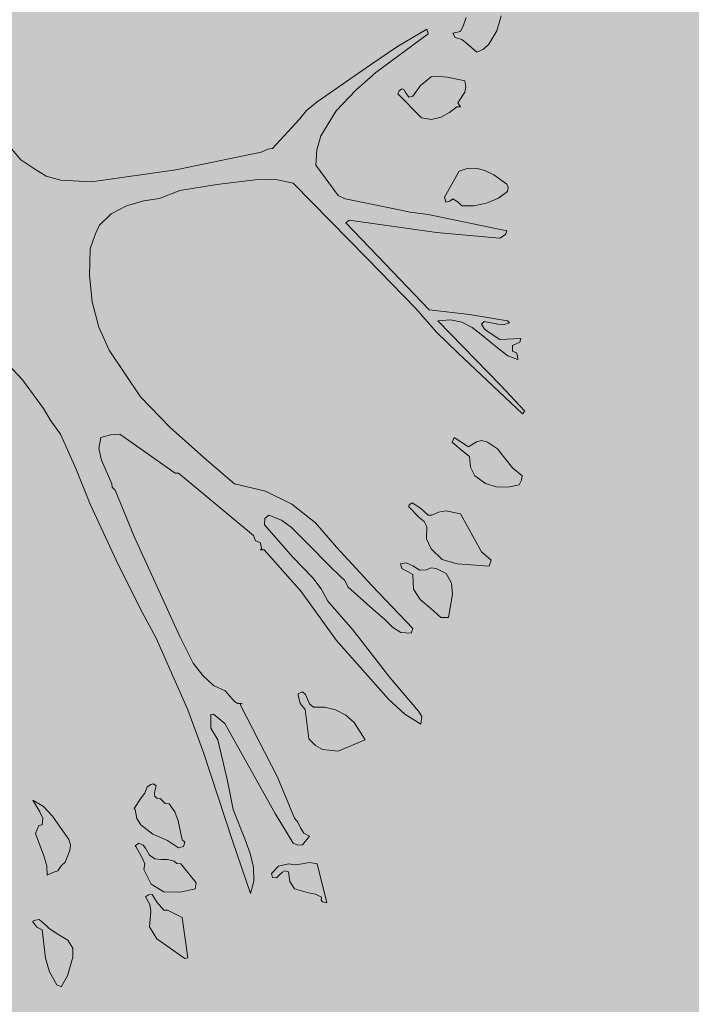
# Model space of a CAD drawing. Units: inches. Extents: x 84 to 1044, y -280 to 906.
# Tile 84 of 105: x 844.48 to 855.93, y 408.65 to 425.45. Entities that reach past the tile are written whole.
import ezdxf

# ---------------------------------------------------------------- set-up
doc = ezdxf.new("R2010")
doc.units = ezdxf.units.IN
doc.layers.add('A-ANNO-DIMS', color=2, linetype='Continuous', lineweight=18)
doc.layers.add('L-PLNT', color=114, linetype='Continuous', lineweight=15)
doc.layers.add('L-PLNT-PATT', color=9, linetype='Continuous', lineweight=9, true_color=0xafd9aa)
doc.styles.get("Standard").update_dxf_attribs({"font": 'arial.ttf'})
doc.dimstyles.get("Standard").update_dxf_attribs({"dimtxt": 0.18, "dimasz": 0.18, "dimexe": 0.18, "dimexo": 0.0625, "dimgap": 0.09, "dimtad": 0, "dimtih": 1, "dimtoh": 1, "dimdec": 4, "dimzin": 0, "dimdsep": 46, "dimtxsty": 'Standard', "dimcen": 0.09, "dimadec": 0, "dimazin": 0, "dimtfac": 1, "dimtdec": 4, "dimtofl": 0, "dimtmove": 0, "dimatfit": 3, "dimfxl": 1, "dimtolj": 1, "dimtzin": 0, "dimarcsym": 0})

# ---------------------------------------------------------------- blocks, each defined once
blk = doc.blocks.new('A$C37E508DF')
for p, q in [((1.3455, 1.0934), (1.3485, 1.102)), ((1.3875, 1.1037), (1.3828, 1.087)), ((1.3057, 1.0835), (1.2469, 1.0402)), ((1.2713, 1.0694), (1.3044, 1.0887)), ((1.3044, 1.0887), (1.3057, 1.0835)), ((1.3335, 1.0844), (1.3421, 1.0861)), ((1.3361, 1.0793), (1.3335, 1.0844)), ((1.3421, 1.0861), (1.3455, 1.0934)), ((1.3828, 1.087), (1.3738, 1.072)), ((1.3434, 1.0771), (1.3361, 1.0793)), ((1.349, 1.0728), (1.3434, 1.0771)), ((1.3605, 1.063), (1.349, 1.0728)), ((1.2409, 1.0488), (1.2713, 1.0694)), ((1.3678, 1.0664), (1.3605, 1.063)), ((1.3738, 1.072), (1.3678, 1.0664)), ((1.1813, 1.0072), (1.2409, 1.0488)), ((1.2469, 1.0402), (1.2246, 1.0201)), ((1.2971, 1.0257), (1.3091, 1.0351)), ((1.3091, 1.0351), (1.3185, 1.0355)), ((1.3185, 1.0355), (1.3275, 1.0347)), ((1.3275, 1.0347), (1.3468, 1.0308)), ((1.3468, 1.0308), (1.3481, 1.0239)), ((1.2246, 1.0201), (1.2023, 0.9969)), ((1.2718, 1.0162), (1.2731, 1.0197)), ((1.2731, 1.0197), (1.2761, 1.0218)), ((1.2761, 1.0218), (1.2786, 1.0209)), ((1.2786, 1.0209), (1.2799, 1.0184)), ((1.2799, 1.0184), (1.2842, 1.0124)), ((1.2885, 1.0136), (1.2971, 1.0257)), ((1.3468, 1.018), (1.3391, 1.0059)), ((1.3481, 1.0239), (1.3468, 1.018)), ((1.1693, 0.9974), (1.1813, 1.0072)), ((1.2984, 0.9892), (1.2718, 1.0162)), ((1.2842, 1.0124), (1.2885, 1.0136)), ((1.3391, 1.0059), (1.3421, 1.0016)), ((1.1612, 0.9879), (1.1693, 0.9974)), ((1.2023, 0.9969), (1.1852, 0.9691)), ((1.3297, 0.9952), (1.3202, 0.9901)), ((1.3378, 1.0016), (1.3297, 0.9952)), ((1.3421, 1.0016), (1.3378, 1.0016)), ((1.1311, 0.9549), (1.1612, 0.9879)), ((1.3095, 0.9875), (1.2984, 0.9892)), ((1.3202, 0.9901), (1.3095, 0.9875)), ((1.1852, 0.9691), (1.1809, 0.9532)), ((0.8383, 0.954), (0.8486, 0.942)), ((1.0227, 0.9309), (1.1183, 0.9506)), ((1.1183, 0.9506), (1.1256, 0.954)), ((1.1256, 0.954), (1.1311, 0.9549)), ((1.1809, 0.9532), (1.1796, 0.936)), ((0.8486, 0.942), (0.8619, 0.933)), ((0.8619, 0.933), (0.8769, 0.9236)), ((0.9279, 0.9172), (1.0227, 0.9309)), ((1.1796, 0.936), (1.2049, 0.9022)), ((1.3241, 0.9), (1.3404, 0.9292)), ((1.3404, 0.9292), (1.3494, 0.9322)), ((1.3494, 0.9322), (1.3592, 0.9326)), ((1.3592, 0.9326), (1.3695, 0.93)), ((1.3695, 0.93), (1.3794, 0.9253)), ((0.8769, 0.9236), (0.8936, 0.9193)), ((0.8936, 0.9193), (0.9279, 0.9172)), ((1.1114, 0.9198), (1.0685, 0.9142)), ((1.1333, 0.9202), (1.1114, 0.9198)), ((1.1543, 0.9159), (1.1333, 0.9202)), ((1.3794, 0.9253), (1.394, 0.9146)), ((1.0269, 0.9077), (1.0042, 0.8987)), ((1.0685, 0.9142), (1.0269, 0.9077)), ((1.2371, 0.8314), (1.1543, 0.9159)), ((1.3948, 0.9065), (1.3846, 0.8992)), ((1.394, 0.9146), (1.3957, 0.9112)), ((1.3957, 0.9112), (1.3948, 0.9065)), ((0.9866, 0.8962), (0.9673, 0.8906)), ((1.0042, 0.8987), (0.9866, 0.8962)), ((1.2049, 0.9022), (1.2126, 0.8983)), ((1.2126, 0.8983), (1.2662, 0.8876)), ((1.3254, 0.8944), (1.3241, 0.9)), ((1.3301, 0.8957), (1.3254, 0.8944)), ((1.3335, 0.8983), (1.3301, 0.8957)), ((1.3395, 0.8944), (1.3335, 0.8983)), ((1.3846, 0.8992), (1.3713, 0.8936)), ((0.9673, 0.8906), (0.9498, 0.8816)), ((1.2662, 0.8876), (1.2855, 0.8833)), ((1.3434, 0.8906), (1.3395, 0.8944)), ((1.3571, 0.8906), (1.3434, 0.8906)), ((1.3713, 0.8936), (1.3571, 0.8906)), ((0.9498, 0.8816), (0.9369, 0.8687)), ((1.2169, 0.8743), (1.2135, 0.8713)), ((1.3151, 0.8606), (1.2169, 0.8743)), ((1.2855, 0.8833), (1.3057, 0.8807)), ((1.3057, 0.8807), (1.394, 0.8623)), ((0.9369, 0.8687), (0.933, 0.861)), ((1.2135, 0.8713), (1.2491, 0.834)), ((1.394, 0.8623), (1.3927, 0.8584)), ((0.9296, 0.852), (0.9262, 0.8421)), ((0.933, 0.861), (0.9296, 0.852)), ((1.3863, 0.8541), (1.3151, 0.8606)), ((1.3927, 0.8584), (1.3863, 0.8541)), ((0.9262, 0.8421), (0.9257, 0.8121)), ((1.2919, 0.7752), (1.2371, 0.8314)), ((1.2491, 0.834), (1.3069, 0.7735)), ((0.9257, 0.8121), (0.9287, 0.7825)), ((0.9287, 0.7825), (0.936, 0.7542)), ((1.3151, 0.7487), (1.2919, 0.7752)), ((1.3069, 0.7735), (1.352, 0.7684)), ((1.352, 0.7684), (1.3948, 0.7615)), ((0.936, 0.7542), (0.9476, 0.7285)), ((1.3309, 0.7624), (1.3164, 0.7615)), ((1.3164, 0.7615), (1.3871, 0.6891)), ((1.3434, 0.7598), (1.3309, 0.7624)), ((1.355, 0.7538), (1.3434, 0.7598)), ((1.3653, 0.7461), (1.355, 0.7538)), ((1.3687, 0.7607), (1.3657, 0.7577)), ((1.3657, 0.7577), (1.3691, 0.7521)), ((1.3841, 0.7577), (1.3687, 0.7607)), ((1.3691, 0.7521), (1.3743, 0.7482)), ((1.3914, 0.7572), (1.3841, 0.7577)), ((1.397, 0.759), (1.3914, 0.7572)), ((1.3948, 0.7615), (1.397, 0.759)), ((1.3391, 0.7255), (1.3151, 0.7487)), ((1.3854, 0.7294), (1.3653, 0.7461)), ((1.3743, 0.7482), (1.3863, 0.7405)), ((1.3863, 0.7405), (1.4099, 0.7414)), ((1.4099, 0.7414), (1.4086, 0.7375)), ((1.4086, 0.7375), (1.4004, 0.7337)), ((1.4004, 0.7337), (1.4004, 0.7272)), ((0.9476, 0.7285), (0.9828, 0.6762)), ((1.4116, 0.6569), (1.3391, 0.7255)), ((1.3953, 0.7221), (1.3854, 0.7294)), ((1.4064, 0.7178), (1.3953, 0.7221)), ((1.4004, 0.7272), (1.4047, 0.7255)), ((1.4047, 0.7255), (1.406, 0.7221)), ((1.406, 0.7221), (1.4064, 0.7178)), ((0.8503, 0.6951), (0.8344, 0.7122)), ((0.8739, 0.6629), (0.8503, 0.6951)), ((1.3871, 0.6891), (1.4141, 0.6599)), ((0.9828, 0.6762), (1.0162, 0.6415)), ((0.8824, 0.6492), (0.8739, 0.6629)), ((1.4141, 0.6599), (1.4116, 0.6569)), ((0.8932, 0.6342), (0.8824, 0.6492)), ((1.0162, 0.6415), (1.0574, 0.605)), ((0.9103, 0.5956), (0.8932, 0.6342)), ((0.9382, 0.6303), (0.936, 0.6179)), ((0.9493, 0.6333), (0.9382, 0.6303)), ((0.9596, 0.6342), (0.9493, 0.6333)), ((1.0218, 0.5904), (0.9596, 0.6342)), ((1.3327, 0.6252), (1.3348, 0.6303)), ((1.3348, 0.6303), (1.3511, 0.62)), ((1.343, 0.6162), (1.3327, 0.6252)), ((1.3511, 0.62), (1.3601, 0.6256)), ((1.3601, 0.6256), (1.3661, 0.6269)), ((1.3661, 0.6269), (1.3725, 0.6252)), ((1.3725, 0.6252), (1.3837, 0.6175)), ((0.936, 0.6179), (0.939, 0.605)), ((1.352, 0.6089), (1.343, 0.6162)), ((1.3533, 0.5969), (1.352, 0.6089)), ((1.3837, 0.6175), (1.3918, 0.6072)), ((0.939, 0.605), (0.9506, 0.5784)), ((1.0574, 0.605), (1.0883, 0.5784)), ((1.358, 0.5874), (1.3533, 0.5969)), ((1.3918, 0.6072), (1.4004, 0.5964)), ((0.9262, 0.5557), (0.9103, 0.5956)), ((1.0256, 0.5904), (1.0218, 0.5904)), ((1.1097, 0.5205), (1.0256, 0.5904)), ((1.37, 0.5789), (1.358, 0.5874)), ((1.4004, 0.5964), (1.4111, 0.5874)), ((1.4111, 0.5874), (1.4103, 0.5823)), ((0.9506, 0.5784), (0.951, 0.5746)), ((1.0883, 0.5784), (1.123, 0.5703)), ((1.3824, 0.575), (1.37, 0.5789)), ((1.3953, 0.5746), (1.3824, 0.575)), ((1.4077, 0.5771), (1.3953, 0.5746)), ((1.4103, 0.5823), (1.4077, 0.5771)), ((0.951, 0.5746), (0.9545, 0.5711)), ((0.9545, 0.5711), (0.9759, 0.5193)), ((1.123, 0.5703), (1.1526, 0.5557)), ((0.9583, 0.4871), (0.9262, 0.5557)), ((1.1526, 0.5557), (1.1792, 0.5347)), ((1.2842, 0.554), (1.2855, 0.5557)), ((1.2842, 0.5527), (1.2842, 0.554)), ((1.2958, 0.5407), (1.2842, 0.5527)), ((1.2855, 0.5557), (1.2876, 0.557)), ((1.2876, 0.557), (1.2971, 0.551)), ((1.1268, 0.5433), (1.1226, 0.5394)), ((1.141, 0.5377), (1.1268, 0.5433)), ((1.2971, 0.551), (1.3057, 0.5433)), ((1.3057, 0.5433), (1.3099, 0.5433)), ((1.3099, 0.5433), (1.3172, 0.5467)), ((1.3172, 0.5467), (1.3254, 0.548)), ((1.3254, 0.548), (1.3421, 0.5446)), ((1.3421, 0.5446), (1.3657, 0.5021)), ((1.1226, 0.5394), (1.1221, 0.5325)), ((1.1221, 0.5325), (1.1539, 0.4961)), ((1.1521, 0.5296), (1.141, 0.5377)), ((1.1792, 0.5347), (1.2027, 0.5072)), ((1.3014, 0.536), (1.2958, 0.5407)), ((1.3044, 0.53), (1.3014, 0.536)), ((1.1118, 0.5145), (1.1097, 0.5205)), ((1.1706, 0.5111), (1.1521, 0.5296)), ((1.3039, 0.5167), (1.3044, 0.53)), ((0.9759, 0.5193), (1.0269, 0.4069)), ((1.117, 0.5124), (1.1118, 0.5145)), ((1.1191, 0.5055), (1.117, 0.5124)), ((1.1955, 0.4858), (1.1706, 0.5111)), ((1.3091, 0.5055), (1.3039, 0.5167)), ((1.117, 0.5042), (1.1191, 0.5055)), ((1.1217, 0.5042), (1.117, 0.5042)), ((1.1633, 0.4575), (1.1217, 0.5042)), ((1.2027, 0.5072), (1.2426, 0.4644)), ((1.3215, 0.4935), (1.3091, 0.5055)), ((1.3657, 0.5021), (1.3764, 0.4927)), ((0.9853, 0.4335), (0.9583, 0.4871)), ((1.1539, 0.4961), (1.1762, 0.4729)), ((1.2748, 0.4884), (1.2812, 0.4897)), ((1.2761, 0.4832), (1.2748, 0.4884)), ((1.2812, 0.4897), (1.2885, 0.4862)), ((1.3382, 0.4884), (1.3215, 0.4935)), ((1.3743, 0.4858), (1.3382, 0.4884)), ((1.3764, 0.4927), (1.3743, 0.4858)), ((1.207, 0.4747), (1.1955, 0.4858)), ((1.2825, 0.4798), (1.2761, 0.4832)), ((1.2885, 0.4764), (1.2825, 0.4798)), ((1.2885, 0.4862), (1.2962, 0.4815)), ((1.2894, 0.4601), (1.2885, 0.4764)), ((1.2962, 0.4815), (1.3039, 0.482)), ((1.3039, 0.482), (1.3087, 0.4841)), ((1.3087, 0.4841), (1.3147, 0.4832)), ((1.3147, 0.4832), (1.3258, 0.4777)), ((1.3258, 0.4777), (1.3318, 0.4669)), ((1.1762, 0.4729), (1.1856, 0.4605)), ((1.2122, 0.47), (1.207, 0.4747)), ((1.2156, 0.4627), (1.2122, 0.47)), ((1.2426, 0.4644), (1.2885, 0.4159)), ((1.3318, 0.4669), (1.3331, 0.4545)), ((1.2027, 0.4026), (1.1633, 0.4575)), ((1.1856, 0.4605), (1.1933, 0.4468)), ((1.2469, 0.4348), (1.2156, 0.4627)), ((1.2967, 0.4485), (1.2894, 0.4601)), ((1.3331, 0.4545), (1.3284, 0.4284)), ((1.1933, 0.4468), (1.2212, 0.4146)), ((1.3082, 0.4386), (1.2967, 0.4485)), ((1.0003, 0.4052), (0.9853, 0.4335)), ((1.2568, 0.4266), (1.2469, 0.4348)), ((1.3198, 0.4284), (1.3082, 0.4386)), ((1.2658, 0.4176), (1.2568, 0.4266)), ((1.3284, 0.4284), (1.3198, 0.4284)), ((1.2212, 0.4146), (1.2628, 0.361)), ((1.2752, 0.4116), (1.2658, 0.4176)), ((1.2868, 0.4108), (1.2752, 0.4116)), ((1.2885, 0.4159), (1.2868, 0.4108)), ((1.0145, 0.373), (1.0003, 0.4052)), ((1.0269, 0.4069), (1.0419, 0.3769)), ((1.2289, 0.373), (1.2027, 0.4026)), ((1.0419, 0.3769), (1.0527, 0.3632)), ((1.0359, 0.3246), (1.0145, 0.373)), ((1.2615, 0.3362), (1.2289, 0.373)), ((1.0527, 0.3632), (1.0647, 0.352)), ((1.2628, 0.361), (1.2949, 0.3233)), ((1.0647, 0.352), (1.078, 0.346)), ((1.078, 0.346), (1.0883, 0.334)), ((1.1599, 0.3426), (1.1646, 0.3447)), ((1.1646, 0.3447), (1.168, 0.3417)), ((1.0883, 0.334), (1.0921, 0.3319)), ((1.0921, 0.3319), (1.0968, 0.3319)), ((1.0968, 0.3319), (1.0947, 0.3306)), ((1.1599, 0.3413), (1.1599, 0.3426)), ((1.162, 0.3319), (1.1599, 0.3413)), ((1.1676, 0.325), (1.162, 0.3319)), ((1.168, 0.3417), (1.1702, 0.3366)), ((1.1702, 0.3366), (1.1727, 0.3314)), ((1.2795, 0.3199), (1.2615, 0.3362)), ((1.0535, 0.2766), (1.0359, 0.3246)), ((1.0947, 0.3306), (1.1367, 0.2491)), ((1.1719, 0.292), (1.1676, 0.325)), ((1.1727, 0.3314), (1.177, 0.3276)), ((1.177, 0.3276), (1.1895, 0.3276)), ((1.1895, 0.3276), (1.2019, 0.3246)), ((1.2019, 0.3246), (1.2135, 0.3186)), ((1.2949, 0.3233), (1.2988, 0.3173)), ((1.0647, 0.3199), (1.0617, 0.3194)), ((1.0617, 0.3194), (1.0617, 0.304)), ((1.0711, 0.3147), (1.0647, 0.3199)), ((1.0775, 0.3092), (1.0711, 0.3147)), ((1.2135, 0.3186), (1.2225, 0.3104)), ((1.2225, 0.3104), (1.2349, 0.2911)), ((1.2975, 0.3087), (1.2795, 0.3199)), ((1.2988, 0.3173), (1.2975, 0.3087)), ((1.0617, 0.304), (1.0698, 0.2911)), ((1.1341, 0.2084), (1.0775, 0.3092)), ((1.0698, 0.2911), (1.0805, 0.2448)), ((1.1792, 0.2847), (1.1719, 0.292)), ((1.2349, 0.2911), (1.2049, 0.2783)), ((1.0861, 0.1775), (1.0535, 0.2766)), ((1.1873, 0.28), (1.1792, 0.2847)), ((1.2049, 0.2783), (1.1873, 0.28)), ((1.0805, 0.2448), (1.087, 0.2127)), ((1.1367, 0.2491), (1.1556, 0.2032)), ((0.9879, 0.2311), (0.9905, 0.2384)), ((0.9905, 0.2384), (0.9943, 0.241)), ((0.9943, 0.241), (0.9973, 0.2414)), ((0.9973, 0.2414), (1.0003, 0.2393)), ((1.0003, 0.2393), (0.9986, 0.232)), ((0.8619, 0.2234), (0.8739, 0.2161)), ((0.87, 0.2101), (0.8619, 0.2234)), ((0.9759, 0.214), (0.9836, 0.226)), ((0.9836, 0.226), (0.9879, 0.2311)), ((0.9986, 0.232), (0.9986, 0.2281)), ((0.9986, 0.2281), (1.0012, 0.2255)), ((1.0012, 0.2255), (1.0051, 0.2251)), ((1.0051, 0.2251), (1.0076, 0.2225)), ((1.0076, 0.2225), (1.0106, 0.2195)), ((0.8734, 0.2032), (0.87, 0.2101)), ((0.8739, 0.2161), (0.8841, 0.2054)), ((0.9768, 0.2127), (0.9759, 0.214)), ((0.9789, 0.2028), (0.9768, 0.2127)), ((1.0106, 0.2195), (1.0149, 0.2191)), ((1.0149, 0.2191), (1.0214, 0.2101)), ((1.0214, 0.2101), (1.0252, 0.2002)), ((1.087, 0.2127), (1.0998, 0.1797)), ((0.8726, 0.1955), (0.8734, 0.2032)), ((0.8841, 0.2054), (0.9026, 0.1792)), ((0.9832, 0.1955), (0.9789, 0.2028)), ((1.0252, 0.2002), (1.0295, 0.1788)), ((1.1543, 0.1749), (1.1341, 0.2084)), ((1.1556, 0.2032), (1.1594, 0.1985)), ((0.8649, 0.1857), (0.8687, 0.1947)), ((0.8687, 0.1947), (0.8726, 0.1955)), ((0.9969, 0.1852), (0.9832, 0.1955)), ((1.1594, 0.1985), (1.1624, 0.1921)), ((1.1624, 0.1921), (1.1663, 0.1861)), ((0.8743, 0.1608), (0.8649, 0.1857)), ((0.9026, 0.1792), (0.9043, 0.1732)), ((1.0132, 0.1779), (0.9969, 0.1852)), ((1.0256, 0.1698), (1.0132, 0.1779)), ((1.0295, 0.1788), (1.0325, 0.1762)), ((1.1063, 0.1183), (1.0861, 0.1775)), ((1.0998, 0.1797), (1.1058, 0.1634)), ((1.1727, 0.1827), (1.1646, 0.1732)), ((1.1663, 0.1861), (1.1727, 0.1827)), ((0.9035, 0.1668), (0.8983, 0.1535)), ((0.9043, 0.1732), (0.9035, 0.1668)), ((0.9768, 0.1719), (0.9811, 0.1749)), ((0.9776, 0.1711), (0.9768, 0.1719)), ((0.9853, 0.1578), (0.9776, 0.1711)), ((0.9811, 0.1749), (0.9858, 0.1728)), ((0.9858, 0.1728), (0.9884, 0.1694)), ((0.9884, 0.1694), (0.9931, 0.1616)), ((1.0312, 0.1711), (1.0256, 0.1698)), ((1.0325, 0.1762), (1.0312, 0.1711)), ((1.1594, 0.1728), (1.1543, 0.1749)), ((1.1646, 0.1732), (1.1594, 0.1728)), ((0.8777, 0.1496), (0.8743, 0.1608)), ((0.9879, 0.1518), (0.9853, 0.1578)), ((0.9931, 0.1616), (0.9991, 0.1574)), ((0.9991, 0.1574), (1.0059, 0.1565)), ((1.0059, 0.1565), (1.0132, 0.1565)), ((1.0132, 0.1565), (1.0205, 0.1548)), ((1.0205, 0.1548), (1.0235, 0.1522)), ((1.1058, 0.1634), (1.1097, 0.1475)), ((0.8781, 0.1389), (0.8777, 0.1496)), ((0.8902, 0.1441), (0.8846, 0.1419)), ((0.894, 0.1496), (0.8902, 0.1441)), ((0.8983, 0.1535), (0.894, 0.1496)), ((0.9866, 0.1453), (0.9879, 0.1518)), ((0.9948, 0.1291), (0.9866, 0.1453)), ((1.0235, 0.1522), (1.0282, 0.1518)), ((1.0282, 0.1518), (1.0454, 0.1303)), ((1.1097, 0.1475), (1.1101, 0.1325)), ((1.1298, 0.1411), (1.1376, 0.1492)), ((1.1376, 0.1492), (1.1491, 0.1518)), ((1.1449, 0.1441), (1.1423, 0.1423)), ((1.1491, 0.1428), (1.1449, 0.1441)), ((1.1491, 0.1518), (1.1564, 0.1505)), ((1.1564, 0.1505), (1.1642, 0.1518)), ((1.1642, 0.1518), (1.1727, 0.1531)), ((1.1727, 0.1531), (1.1813, 0.1518)), ((1.1813, 0.1518), (1.192, 0.108)), ((0.8846, 0.1419), (0.8781, 0.1389)), ((1.1311, 0.1364), (1.1298, 0.1411)), ((1.1354, 0.1359), (1.1311, 0.1364)), ((1.1384, 0.1389), (1.1354, 0.1359)), ((1.1423, 0.1423), (1.1384, 0.1389)), ((1.1504, 0.132), (1.1491, 0.1428)), ((1.0089, 0.1205), (0.9948, 0.1291)), ((1.0441, 0.1239), (1.0274, 0.12)), ((1.0454, 0.1303), (1.0441, 0.1239)), ((1.1101, 0.1325), (1.1063, 0.1183)), ((1.1556, 0.1239), (1.1504, 0.132)), ((1.1714, 0.1192), (1.1556, 0.1239)), ((0.9884, 0.1149), (0.9918, 0.117)), ((0.9935, 0.1063), (0.9884, 0.1149)), ((0.9918, 0.117), (0.9961, 0.1175)), ((0.9961, 0.1175), (1.0016, 0.1085)), ((1.0274, 0.12), (1.0089, 0.1205)), ((1.1792, 0.1179), (1.1714, 0.1192)), ((1.186, 0.1145), (1.1792, 0.1179)), ((1.1856, 0.111), (1.186, 0.1145)), ((1.1873, 0.1093), (1.1856, 0.111)), ((0.9943, 0.0982), (0.9935, 0.1063)), ((1.0016, 0.1085), (1.0089, 0.0999)), ((1.0089, 0.0999), (1.0132, 0.0999)), ((1.0132, 0.0999), (1.0295, 0.0917)), ((1.192, 0.108), (1.1873, 0.1093)), ((0.8619, 0.0875), (0.8649, 0.0887)), ((0.8649, 0.0887), (0.8691, 0.0892)), ((0.8691, 0.0892), (0.8769, 0.0827)), ((0.9931, 0.081), (0.9943, 0.0982)), ((1.0295, 0.0917), (1.0359, 0.0463)), ((0.8619, 0.0866), (0.8619, 0.0875)), ((0.8666, 0.0806), (0.8619, 0.0866)), ((0.8726, 0.0776), (0.8666, 0.0806)), ((0.8764, 0.0459), (0.8726, 0.0776)), ((0.8769, 0.0827), (0.8799, 0.0797)), ((0.8799, 0.0797), (0.8893, 0.0733)), ((1.0012, 0.0677), (0.9931, 0.081)), ((0.8893, 0.0733), (0.9013, 0.066)), ((1.0325, 0.0454), (1.0012, 0.0677)), ((0.9013, 0.066), (0.9069, 0.057)), ((0.9069, 0.057), (0.9069, 0.0471)), ((0.8807, 0.0304), (0.8764, 0.0459)), ((0.9069, 0.0471), (0.9009, 0.0261)), ((1.0359, 0.0463), (1.0325, 0.0454)), ((0.8889, 0.0159), (0.8807, 0.0304)), ((0.9009, 0.0261), (0.894, 0.0137)), ((0.894, 0.0137), (0.8889, 0.0159))]:
    blk.add_line(p, q)
blk = doc.blocks.new('*D62')
at = {"layer": 'A-ANNO-DIMS', "color": 0, "lineweight": -2, "transparency": 16777216}
for p, q in [((203.179, 709.183), (203.179, 905.9)), ((896.074, 400.183), (896.074, 905.9)), ((203.359, 905.72), (549.232, 905.72)), ((895.894, 905.72), (550.021, 905.72))]:
    blk.add_line(p, q, dxfattribs=at)
at = {"layer": 'A-ANNO-DIMS', "color": 0, "transparency": 16777216}
for points in [[(203.359, 905.75), (203.359, 905.69), (203.179, 905.72)], [(895.894, 905.75), (895.894, 905.69), (896.074, 905.72)]]:
    blk.add_solid(points, dxfattribs=at)
at = {"layer": 'Defpoints', "color": 0, "transparency": 16777216}
for p in [(896.074, 905.72), (203.179, 709.12), (896.074, 400.12)]:
    blk.add_point(p, dxfattribs=at)
at = {"layer": 'A-ANNO-DIMS', "color": 0, "transparency": 16777216, "insert": (549.627, 905.72), "char_height": 0.18, "attachment_point": 5}
blk.add_mtext('\\A1;692.9', dxfattribs=at)
blk = doc.blocks.new('*D63')
at = {"layer": 'A-ANNO-DIMS', "color": 0, "lineweight": -2, "transparency": 16777216}
for p, q in [((833.136, 709.12), (1043.768, 709.12)), ((1043.588, 708.94), (1043.588, 400.302)), ((1043.588, 91.3), (1043.588, 399.938)), ((896.136, 91.12), (1043.768, 91.12))]:
    blk.add_line(p, q, dxfattribs=at)
at = {"layer": 'A-ANNO-DIMS', "color": 0, "transparency": 16777216}
for points in [[(1043.558, 708.94), (1043.618, 708.94), (1043.588, 709.12)], [(1043.558, 91.3), (1043.618, 91.3), (1043.588, 91.12)]]:
    blk.add_solid(points, dxfattribs=at)
at = {"layer": 'Defpoints', "color": 0, "transparency": 16777216}
for p in [(833.074, 709.12), (1043.588, 709.12), (896.074, 91.12)]:
    blk.add_point(p, dxfattribs=at)
at = {"layer": 'A-ANNO-DIMS', "color": 0, "transparency": 16777216, "insert": (1043.588, 400.12), "char_height": 0.18, "attachment_point": 5}
blk.add_mtext('\\A1;618', dxfattribs=at)

msp = doc.modelspace()

# ---------------------------------------------------------------- hatches: boundary and pattern name
at = {"layer": 'L-PLNT-PATT', "transparency": 33554597}
h = msp.add_hatch(color=256, dxfattribs=at)
h.dxf.hatch_style = 1
h.paths.add_polyline_path([(896.074, 511.12), (704.074, 511.12), (704.074, 491.62), (704.074, 419.62), (704.074, 400.12), (833.074, 400.12), (896.074, 400.12)])

# ---------------------------------------------------------------- block references
at = {"layer": 'L-PLNT', "xscale": 15.19586232982809, "yscale": 15.19586232982809, "zscale": 15.19586232982809}
msp.add_blockref('A$C37E508DF', (831.605, 408.742), dxfattribs=at)

# ---------------------------------------------------------------- dimensions: what is measured, and where the dimension line sits
at = {"layer": 'A-ANNO-DIMS'}
dim = msp.add_linear_dim(base=(896.074, 905.72), p1=(203.179, 709.12), p2=(896.074, 400.12), dimstyle='Standard', override={"dimdec": 1, "dimlfac": 1, "dimrnd": 0, "dimzin": 0, "dimdsep": 46, "dimlunit": 2}, dxfattribs=at)
dim.commit()
dim.dimension.update_dxf_attribs({"geometry": '*D62', "text_midpoint": (549.627, 905.72)})
dim = msp.add_linear_dim(base=(1043.588, 709.12), p1=(896.074, 91.12), p2=(833.074, 709.12), angle=90, dimstyle='Standard', override={"dimdec": 0, "dimlfac": 1, "dimrnd": 0, "dimzin": 0, "dimdsep": 46, "dimlunit": 2}, dxfattribs=at)
dim.commit()
dim.dimension.update_dxf_attribs({"geometry": '*D63', "text_midpoint": (1043.588, 400.12)})

doc.saveas('drawing.dxf')
